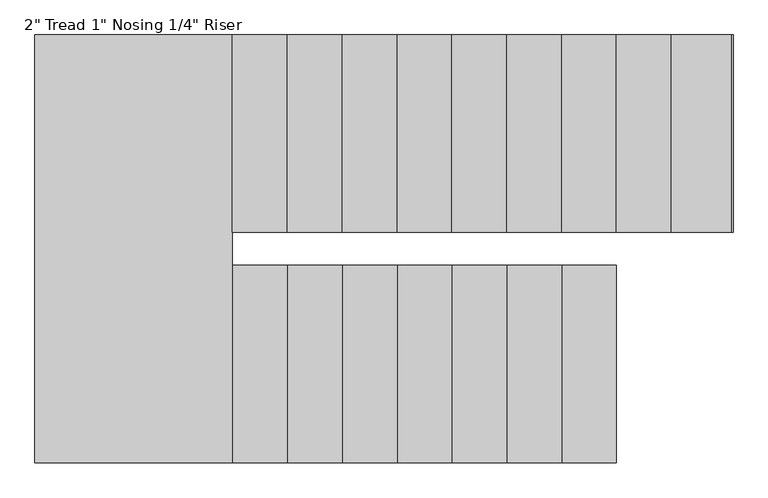
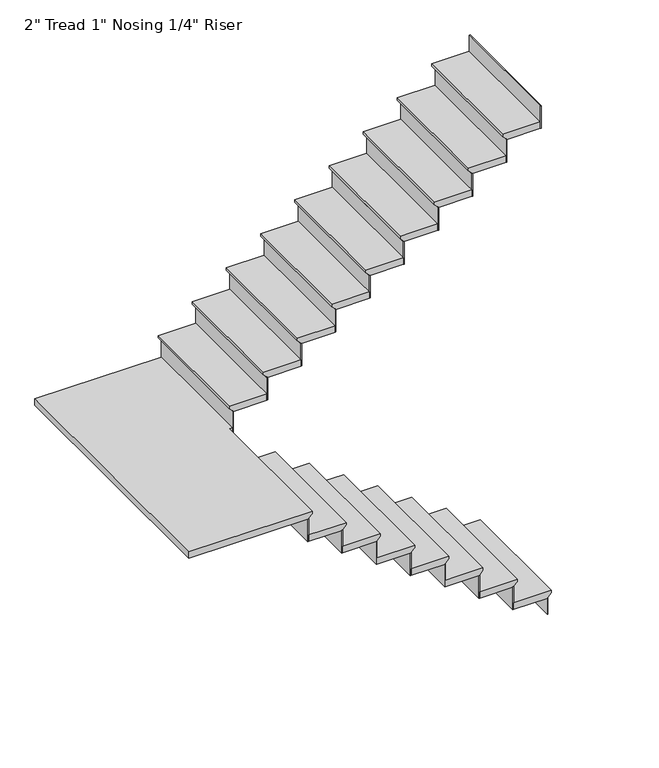
"""IFC4 building model written with IfcOpenShell, lengths in millimetres: stair flight geometry."""

from ifc_helpers import new_model, si_unit, origin, place, context, project, spatial, faceted_brep, source, transform, mapped, element, save


def stair_flight_30e1afdc(model_context):
    return source(origin(), model_context, "Body", "Brep", [
        faceted_brep([(-5739.8201068, -2431.6122986, 158.75), (-5739.8201068, -2431.6122986, 177.8), (-5739.8201068, -3346.0122986, 177.8), (-5739.8201068, -3346.0122986, 158.75), (-5765.2201068, -2431.6122986, 133.35), (-5765.2201068, -3346.0122986, 133.35), (-6019.2201068, -2431.6122986, 177.8), (-6019.2201068, -3346.0122986, 177.8), (-5765.2201068, -3346.0122986, 127.0), (-6019.2201068, -3346.0122986, 127.0), (-6019.2201068, -2431.6122986, 127.0), (-5765.2201068, -2431.6122986, 127.0)], [[[0, 1, 2, 3]], [[4, 0, 3, 5]], [[2, 1, 6, 7]], [[8, 9, 10, 11]], [[2, 7, 9, 8, 5, 3]], [[8, 11, 4, 5]], [[6, 1, 0, 4, 11, 10]], [[7, 6, 10, 9]]]),
        faceted_brep([(-5765.2201068, -2431.6122986, 127.0), (-5765.2201068, -2431.6122986, 0.0), (-5771.5701068, -2431.6122986, 0.0), (-5771.5701068, -2431.6122986, 127.0), (-5765.2201068, -3346.0122986, 127.0), (-5771.5701068, -3346.0122986, 127.0), (-5771.5701068, -3346.0122986, 0.0), (-5765.2201068, -3346.0122986, 0.0)], [[[0, 1, 2, 3]], [[4, 5, 6, 7]], [[1, 0, 4, 7]], [[2, 1, 7, 6]], [[3, 2, 6, 5]], [[0, 3, 5, 4]]]),
        faceted_brep([(-6019.2201068, -2431.6122986, 304.8), (-6019.2201068, -2431.6122986, 127.0), (-6025.5701068, -2431.6122986, 127.0), (-6025.5701068, -2431.6122986, 304.8), (-6019.2201068, -3346.0122986, 304.8), (-6025.5701068, -3346.0122986, 304.8), (-6025.5701068, -3346.0122986, 127.0), (-6019.2201068, -3346.0122986, 127.0)], [[[0, 1, 2, 3]], [[4, 5, 6, 7]], [[1, 0, 4, 7]], [[2, 1, 7, 6]], [[3, 2, 6, 5]], [[0, 3, 5, 4]]]),
        faceted_brep([(-5993.8201068, -3346.0122986, 355.6), (-5993.8201068, -2431.6122986, 355.6), (-6273.2201068, -2431.6122986, 355.6), (-6273.2201068, -3346.0122986, 355.6), (-6019.2201068, -3346.0122986, 304.8), (-6273.2201068, -3346.0122986, 304.8), (-6273.2201068, -2431.6122986, 304.8), (-6019.2201068, -2431.6122986, 304.8), (-6019.2201068, -3346.0122986, 311.15), (-5993.8201068, -3346.0122986, 336.55), (-6019.2201068, -2431.6122986, 311.15), (-5993.8201068, -2431.6122986, 336.55)], [[[0, 1, 2, 3]], [[4, 5, 6, 7]], [[0, 3, 5, 4, 8, 9]], [[4, 7, 10, 8]], [[2, 1, 11, 10, 7, 6]], [[3, 2, 6, 5]], [[11, 1, 0, 9]], [[10, 11, 9, 8]]]),
        faceted_brep([(-6273.2201068, -2431.6122986, 482.6), (-6273.2201068, -2431.6122986, 304.8), (-6279.5701068, -2431.6122986, 304.8), (-6279.5701068, -2431.6122986, 482.6), (-6273.2201068, -3346.0122986, 482.6), (-6279.5701068, -3346.0122986, 482.6), (-6279.5701068, -3346.0122986, 304.8), (-6273.2201068, -3346.0122986, 304.8)], [[[0, 1, 2, 3]], [[4, 5, 6, 7]], [[1, 0, 4, 7]], [[2, 1, 7, 6]], [[3, 2, 6, 5]], [[0, 3, 5, 4]]]),
        faceted_brep([(-6247.8201068, -3346.0122986, 533.4), (-6247.8201068, -2431.6122986, 533.4), (-6527.2201068, -2431.6122986, 533.4), (-6527.2201068, -3346.0122986, 533.4), (-6273.2201068, -3346.0122986, 482.6), (-6527.2201068, -3346.0122986, 482.6), (-6527.2201068, -2431.6122986, 482.6), (-6273.2201068, -2431.6122986, 482.6), (-6273.2201068, -3346.0122986, 488.95), (-6247.8201068, -3346.0122986, 514.35), (-6273.2201068, -2431.6122986, 488.95), (-6247.8201068, -2431.6122986, 514.35)], [[[0, 1, 2, 3]], [[4, 5, 6, 7]], [[0, 3, 5, 4, 8, 9]], [[4, 7, 10, 8]], [[2, 1, 11, 10, 7, 6]], [[3, 2, 6, 5]], [[11, 1, 0, 9]], [[10, 11, 9, 8]]]),
        faceted_brep([(-6527.2201068, -2431.6122986, 660.4), (-6527.2201068, -2431.6122986, 482.6), (-6533.5701068, -2431.6122986, 482.6), (-6533.5701068, -2431.6122986, 660.4), (-6527.2201068, -3346.0122986, 660.4), (-6533.5701068, -3346.0122986, 660.4), (-6533.5701068, -3346.0122986, 482.6), (-6527.2201068, -3346.0122986, 482.6)], [[[0, 1, 2, 3]], [[4, 5, 6, 7]], [[1, 0, 4, 7]], [[2, 1, 7, 6]], [[3, 2, 6, 5]], [[0, 3, 5, 4]]]),
        faceted_brep([(-6501.8201068, -3346.0122986, 711.2), (-6501.8201068, -2431.6122986, 711.2), (-6781.2201068, -2431.6122986, 711.2), (-6781.2201068, -3346.0122986, 711.2), (-6527.2201068, -3346.0122986, 660.4), (-6781.2201068, -3346.0122986, 660.4), (-6781.2201068, -2431.6122986, 660.4), (-6527.2201068, -2431.6122986, 660.4), (-6527.2201068, -3346.0122986, 666.75), (-6501.8201068, -3346.0122986, 692.15), (-6527.2201068, -2431.6122986, 666.75), (-6501.8201068, -2431.6122986, 692.15)], [[[0, 1, 2, 3]], [[4, 5, 6, 7]], [[0, 3, 5, 4, 8, 9]], [[4, 7, 10, 8]], [[2, 1, 11, 10, 7, 6]], [[3, 2, 6, 5]], [[11, 1, 0, 9]], [[10, 11, 9, 8]]]),
        faceted_brep([(-6781.2201068, -2431.6122986, 838.2), (-6781.2201068, -2431.6122986, 660.4), (-6787.5701068, -2431.6122986, 660.4), (-6787.5701068, -2431.6122986, 838.2), (-6781.2201068, -3346.0122986, 838.2), (-6787.5701068, -3346.0122986, 838.2), (-6787.5701068, -3346.0122986, 660.4), (-6781.2201068, -3346.0122986, 660.4)], [[[0, 1, 2, 3]], [[4, 5, 6, 7]], [[1, 0, 4, 7]], [[2, 1, 7, 6]], [[3, 2, 6, 5]], [[0, 3, 5, 4]]]),
        faceted_brep([(-6755.8201068, -3346.0122986, 889.0), (-6755.8201068, -2431.6122986, 889.0), (-7035.2201068, -2431.6122986, 889.0), (-7035.2201068, -3346.0122986, 889.0), (-6781.2201068, -3346.0122986, 838.2), (-7035.2201068, -3346.0122986, 838.2), (-7035.2201068, -2431.6122986, 838.2), (-6781.2201068, -2431.6122986, 838.2), (-6781.2201068, -3346.0122986, 844.55), (-6755.8201068, -3346.0122986, 869.95), (-6781.2201068, -2431.6122986, 844.55), (-6755.8201068, -2431.6122986, 869.95)], [[[0, 1, 2, 3]], [[4, 5, 6, 7]], [[0, 3, 5, 4, 8, 9]], [[4, 7, 10, 8]], [[2, 1, 11, 10, 7, 6]], [[3, 2, 6, 5]], [[11, 1, 0, 9]], [[10, 11, 9, 8]]]),
        faceted_brep([(-7035.2201068, -2431.6122986, 1016.0), (-7035.2201068, -2431.6122986, 838.2), (-7041.5701068, -2431.6122986, 838.2), (-7041.5701068, -2431.6122986, 1016.0), (-7035.2201068, -3346.0122986, 1016.0), (-7041.5701068, -3346.0122986, 1016.0), (-7041.5701068, -3346.0122986, 838.2), (-7035.2201068, -3346.0122986, 838.2)], [[[0, 1, 2, 3]], [[4, 5, 6, 7]], [[1, 0, 4, 7]], [[2, 1, 7, 6]], [[3, 2, 6, 5]], [[0, 3, 5, 4]]]),
        faceted_brep([(-7009.8201068, -3346.0122986, 1066.8), (-7009.8201068, -2431.6122986, 1066.8), (-7289.2201068, -2431.6122986, 1066.8), (-7289.2201068, -3346.0122986, 1066.8), (-7035.2201068, -3346.0122986, 1016.0), (-7289.2201068, -3346.0122986, 1016.0), (-7289.2201068, -2431.6122986, 1016.0), (-7035.2201068, -2431.6122986, 1016.0), (-7035.2201068, -3346.0122986, 1022.35), (-7009.8201068, -3346.0122986, 1047.75), (-7035.2201068, -2431.6122986, 1022.35), (-7009.8201068, -2431.6122986, 1047.75)], [[[0, 1, 2, 3]], [[4, 5, 6, 7]], [[0, 3, 5, 4, 8, 9]], [[4, 7, 10, 8]], [[2, 1, 11, 10, 7, 6]], [[3, 2, 6, 5]], [[11, 1, 0, 9]], [[10, 11, 9, 8]]]),
        faceted_brep([(-7543.2201068, -2431.6122986, 1371.6), (-7543.2201068, -2431.6122986, 1193.8), (-7549.5701068, -2431.6122986, 1193.8), (-7549.5701068, -2431.6122986, 1371.6), (-7543.2201068, -3346.0122986, 1371.6), (-7549.5701068, -3346.0122986, 1371.6), (-7549.5701068, -3346.0122986, 1193.8), (-7543.2201068, -3346.0122986, 1193.8)], [[[0, 1, 2, 3]], [[4, 5, 6, 7]], [[1, 0, 4, 7]], [[2, 1, 7, 6]], [[3, 2, 6, 5]], [[0, 3, 5, 4]]]),
        faceted_brep([(-7492.4201068, -1364.8122986, 1422.4), (-8432.2201068, -1364.8122986, 1422.4), (-8432.2201068, -3346.0122986, 1422.4), (-7517.8201068, -3346.0122986, 1422.4), (-7517.8201068, -2279.2122986, 1422.4), (-7492.4201068, -2279.2122986, 1422.4), (-8432.2201068, -1364.8122986, 1371.6), (-7492.4201068, -1364.8122986, 1371.6), (-7492.4201068, -2279.2122986, 1371.6), (-7517.8201068, -2279.2122986, 1371.6), (-7517.8201068, -2431.6122986, 1371.6), (-7543.2201068, -2431.6122986, 1371.6), (-7543.2201068, -3346.0122986, 1371.6), (-8432.2201068, -3346.0122986, 1371.6), (-7543.2201068, -2431.6122986, 1377.95), (-7543.2201068, -3346.0122986, 1377.95), (-7517.8201068, -3346.0122986, 1403.35), (-7517.8201068, -2431.6122986, 1403.35)], [[[0, 1, 2, 3, 4, 5]], [[6, 7, 8, 9, 10, 11, 12, 13]], [[1, 0, 7, 6]], [[12, 11, 14, 15]], [[4, 3, 16, 17, 10, 9]], [[0, 5, 8, 7]], [[16, 15, 14, 17]], [[2, 1, 6, 13]], [[3, 2, 13, 12, 15, 16]], [[11, 10, 17, 14]], [[5, 4, 9, 8]]]),
        faceted_brep([(-7289.2201068, -2431.6122986, 1193.8), (-7289.2201068, -2431.6122986, 1016.0), (-7295.5701068, -2431.6122986, 1016.0), (-7295.5701068, -2431.6122986, 1193.8), (-7289.2201068, -3346.0122986, 1193.8), (-7295.5701068, -3346.0122986, 1193.8), (-7295.5701068, -3346.0122986, 1016.0), (-7289.2201068, -3346.0122986, 1016.0)], [[[0, 1, 2, 3]], [[4, 5, 6, 7]], [[1, 0, 4, 7]], [[2, 1, 7, 6]], [[3, 2, 6, 5]], [[0, 3, 5, 4]]]),
        faceted_brep([(-7263.8201068, -3346.0122986, 1244.6), (-7263.8201068, -2431.6122986, 1244.6), (-7543.2201068, -2431.6122986, 1244.6), (-7543.2201068, -3346.0122986, 1244.6), (-7289.2201068, -3346.0122986, 1193.8), (-7543.2201068, -3346.0122986, 1193.8), (-7543.2201068, -2431.6122986, 1193.8), (-7289.2201068, -2431.6122986, 1193.8), (-7289.2201068, -3346.0122986, 1200.15), (-7263.8201068, -3346.0122986, 1225.55), (-7289.2201068, -2431.6122986, 1200.15), (-7263.8201068, -2431.6122986, 1225.55)], [[[0, 1, 2, 3]], [[4, 5, 6, 7]], [[0, 3, 5, 4, 8, 9]], [[4, 7, 10, 8]], [[2, 1, 11, 10, 7, 6]], [[3, 2, 6, 5]], [[11, 1, 0, 9]], [[10, 11, 9, 8]]]),
        faceted_brep([(-7492.4201068, -2279.2122986, 1549.4), (-7492.4201068, -2279.2122986, 1371.6), (-7486.0701068, -2279.2122986, 1371.6), (-7486.0701068, -2279.2122986, 1549.4), (-7492.4201068, -1364.8122986, 1549.4), (-7486.0701068, -1364.8122986, 1549.4), (-7486.0701068, -1364.8122986, 1371.6), (-7492.4201068, -1364.8122986, 1371.6)], [[[0, 1, 2, 3]], [[4, 5, 6, 7]], [[1, 0, 4, 7]], [[2, 1, 7, 6]], [[3, 2, 6, 5]], [[0, 3, 5, 4]]]),
        faceted_brep([(-7517.8201068, -1364.8122986, 1600.2), (-7517.8201068, -2279.2122986, 1600.2), (-7238.4201068, -2279.2122986, 1600.2), (-7238.4201068, -1364.8122986, 1600.2), (-7492.4201068, -1364.8122986, 1549.4), (-7238.4201068, -1364.8122986, 1549.4), (-7238.4201068, -2279.2122986, 1549.4), (-7492.4201068, -2279.2122986, 1549.4), (-7492.4201068, -1364.8122986, 1555.75), (-7517.8201068, -1364.8122986, 1581.15), (-7492.4201068, -2279.2122986, 1555.75), (-7517.8201068, -2279.2122986, 1581.15)], [[[0, 1, 2, 3]], [[4, 5, 6, 7]], [[0, 3, 5, 4, 8, 9]], [[4, 7, 10, 8]], [[2, 1, 11, 10, 7, 6]], [[3, 2, 6, 5]], [[11, 1, 0, 9]], [[10, 11, 9, 8]]]),
        faceted_brep([(-7238.4201068, -2279.2122986, 1727.2), (-7238.4201068, -2279.2122986, 1549.4), (-7232.0701068, -2279.2122986, 1549.4), (-7232.0701068, -2279.2122986, 1727.2), (-7238.4201068, -1364.8122986, 1727.2), (-7232.0701068, -1364.8122986, 1727.2), (-7232.0701068, -1364.8122986, 1549.4), (-7238.4201068, -1364.8122986, 1549.4)], [[[0, 1, 2, 3]], [[4, 5, 6, 7]], [[1, 0, 4, 7]], [[2, 1, 7, 6]], [[3, 2, 6, 5]], [[0, 3, 5, 4]]]),
        faceted_brep([(-7263.8201068, -1364.8122986, 1778.0), (-7263.8201068, -2279.2122986, 1778.0), (-6984.4201068, -2279.2122986, 1778.0), (-6984.4201068, -1364.8122986, 1778.0), (-7238.4201068, -1364.8122986, 1727.2), (-6984.4201068, -1364.8122986, 1727.2), (-6984.4201068, -2279.2122986, 1727.2), (-7238.4201068, -2279.2122986, 1727.2), (-7238.4201068, -1364.8122986, 1733.55), (-7263.8201068, -1364.8122986, 1758.95), (-7238.4201068, -2279.2122986, 1733.55), (-7263.8201068, -2279.2122986, 1758.95)], [[[0, 1, 2, 3]], [[4, 5, 6, 7]], [[0, 3, 5, 4, 8, 9]], [[4, 7, 10, 8]], [[2, 1, 11, 10, 7, 6]], [[3, 2, 6, 5]], [[11, 1, 0, 9]], [[10, 11, 9, 8]]]),
        faceted_brep([(-6984.4201068, -2279.2122986, 1905.0), (-6984.4201068, -2279.2122986, 1727.2), (-6978.0701068, -2279.2122986, 1727.2), (-6978.0701068, -2279.2122986, 1905.0), (-6984.4201068, -1364.8122986, 1905.0), (-6978.0701068, -1364.8122986, 1905.0), (-6978.0701068, -1364.8122986, 1727.2), (-6984.4201068, -1364.8122986, 1727.2)], [[[0, 1, 2, 3]], [[4, 5, 6, 7]], [[1, 0, 4, 7]], [[2, 1, 7, 6]], [[3, 2, 6, 5]], [[0, 3, 5, 4]]]),
        faceted_brep([(-7009.8201068, -1364.8122986, 1955.8), (-7009.8201068, -2279.2122986, 1955.8), (-6730.4201068, -2279.2122986, 1955.8), (-6730.4201068, -1364.8122986, 1955.8), (-6984.4201068, -1364.8122986, 1905.0), (-6730.4201068, -1364.8122986, 1905.0), (-6730.4201068, -2279.2122986, 1905.0), (-6984.4201068, -2279.2122986, 1905.0), (-6984.4201068, -1364.8122986, 1911.35), (-7009.8201068, -1364.8122986, 1936.75), (-6984.4201068, -2279.2122986, 1911.35), (-7009.8201068, -2279.2122986, 1936.75)], [[[0, 1, 2, 3]], [[4, 5, 6, 7]], [[0, 3, 5, 4, 8, 9]], [[4, 7, 10, 8]], [[2, 1, 11, 10, 7, 6]], [[3, 2, 6, 5]], [[11, 1, 0, 9]], [[10, 11, 9, 8]]]),
        faceted_brep([(-6730.4201068, -2279.2122986, 2082.8), (-6730.4201068, -2279.2122986, 1905.0), (-6724.0701068, -2279.2122986, 1905.0), (-6724.0701068, -2279.2122986, 2082.8), (-6730.4201068, -1364.8122986, 2082.8), (-6724.0701068, -1364.8122986, 2082.8), (-6724.0701068, -1364.8122986, 1905.0), (-6730.4201068, -1364.8122986, 1905.0)], [[[0, 1, 2, 3]], [[4, 5, 6, 7]], [[1, 0, 4, 7]], [[2, 1, 7, 6]], [[3, 2, 6, 5]], [[0, 3, 5, 4]]]),
        faceted_brep([(-6755.8201068, -1364.8122986, 2133.6), (-6755.8201068, -2279.2122986, 2133.6), (-6476.4201068, -2279.2122986, 2133.6), (-6476.4201068, -1364.8122986, 2133.6), (-6730.4201068, -1364.8122986, 2082.8), (-6476.4201068, -1364.8122986, 2082.8), (-6476.4201068, -2279.2122986, 2082.8), (-6730.4201068, -2279.2122986, 2082.8), (-6730.4201068, -1364.8122986, 2089.15), (-6755.8201068, -1364.8122986, 2114.55), (-6730.4201068, -2279.2122986, 2089.15), (-6755.8201068, -2279.2122986, 2114.55)], [[[0, 1, 2, 3]], [[4, 5, 6, 7]], [[0, 3, 5, 4, 8, 9]], [[4, 7, 10, 8]], [[2, 1, 11, 10, 7, 6]], [[3, 2, 6, 5]], [[11, 1, 0, 9]], [[10, 11, 9, 8]]]),
        faceted_brep([(-6476.4201068, -2279.2122986, 2260.6), (-6476.4201068, -2279.2122986, 2082.8), (-6470.0701068, -2279.2122986, 2082.8), (-6470.0701068, -2279.2122986, 2260.6), (-6476.4201068, -1364.8122986, 2260.6), (-6470.0701068, -1364.8122986, 2260.6), (-6470.0701068, -1364.8122986, 2082.8), (-6476.4201068, -1364.8122986, 2082.8)], [[[0, 1, 2, 3]], [[4, 5, 6, 7]], [[1, 0, 4, 7]], [[2, 1, 7, 6]], [[3, 2, 6, 5]], [[0, 3, 5, 4]]]),
        faceted_brep([(-6501.8201068, -1364.8122986, 2311.4), (-6501.8201068, -2279.2122986, 2311.4), (-6222.4201068, -2279.2122986, 2311.4), (-6222.4201068, -1364.8122986, 2311.4), (-6476.4201068, -1364.8122986, 2260.6), (-6222.4201068, -1364.8122986, 2260.6), (-6222.4201068, -2279.2122986, 2260.6), (-6476.4201068, -2279.2122986, 2260.6), (-6476.4201068, -1364.8122986, 2266.95), (-6501.8201068, -1364.8122986, 2292.35), (-6476.4201068, -2279.2122986, 2266.95), (-6501.8201068, -2279.2122986, 2292.35)], [[[0, 1, 2, 3]], [[4, 5, 6, 7]], [[0, 3, 5, 4, 8, 9]], [[4, 7, 10, 8]], [[2, 1, 11, 10, 7, 6]], [[3, 2, 6, 5]], [[11, 1, 0, 9]], [[10, 11, 9, 8]]]),
        faceted_brep([(-6222.4201068, -2279.2122986, 2438.4), (-6222.4201068, -2279.2122986, 2260.6), (-6216.0701068, -2279.2122986, 2260.6), (-6216.0701068, -2279.2122986, 2438.4), (-6222.4201068, -1364.8122986, 2438.4), (-6216.0701068, -1364.8122986, 2438.4), (-6216.0701068, -1364.8122986, 2260.6), (-6222.4201068, -1364.8122986, 2260.6)], [[[0, 1, 2, 3]], [[4, 5, 6, 7]], [[1, 0, 4, 7]], [[2, 1, 7, 6]], [[3, 2, 6, 5]], [[0, 3, 5, 4]]]),
        faceted_brep([(-6247.8201068, -1364.8122986, 2489.2), (-6247.8201068, -2279.2122986, 2489.2), (-5968.4201068, -2279.2122986, 2489.2), (-5968.4201068, -1364.8122986, 2489.2), (-6222.4201068, -1364.8122986, 2438.4), (-5968.4201068, -1364.8122986, 2438.4), (-5968.4201068, -2279.2122986, 2438.4), (-6222.4201068, -2279.2122986, 2438.4), (-6222.4201068, -1364.8122986, 2444.75), (-6247.8201068, -1364.8122986, 2470.15), (-6222.4201068, -2279.2122986, 2444.75), (-6247.8201068, -2279.2122986, 2470.15)], [[[0, 1, 2, 3]], [[4, 5, 6, 7]], [[0, 3, 5, 4, 8, 9]], [[4, 7, 10, 8]], [[2, 1, 11, 10, 7, 6]], [[3, 2, 6, 5]], [[11, 1, 0, 9]], [[10, 11, 9, 8]]]),
        faceted_brep([(-5968.4201068, -2279.2122986, 2616.2), (-5968.4201068, -2279.2122986, 2438.4), (-5962.0701068, -2279.2122986, 2438.4), (-5962.0701068, -2279.2122986, 2616.2), (-5968.4201068, -1364.8122986, 2616.2), (-5962.0701068, -1364.8122986, 2616.2), (-5962.0701068, -1364.8122986, 2438.4), (-5968.4201068, -1364.8122986, 2438.4)], [[[0, 1, 2, 3]], [[4, 5, 6, 7]], [[1, 0, 4, 7]], [[2, 1, 7, 6]], [[3, 2, 6, 5]], [[0, 3, 5, 4]]]),
        faceted_brep([(-5993.8201068, -1364.8122986, 2667.0), (-5993.8201068, -2279.2122986, 2667.0), (-5714.4201068, -2279.2122986, 2667.0), (-5714.4201068, -1364.8122986, 2667.0), (-5968.4201068, -1364.8122986, 2616.2), (-5714.4201068, -1364.8122986, 2616.2), (-5714.4201068, -2279.2122986, 2616.2), (-5968.4201068, -2279.2122986, 2616.2), (-5968.4201068, -1364.8122986, 2622.55), (-5993.8201068, -1364.8122986, 2647.95), (-5968.4201068, -2279.2122986, 2622.55), (-5993.8201068, -2279.2122986, 2647.95)], [[[0, 1, 2, 3]], [[4, 5, 6, 7]], [[0, 3, 5, 4, 8, 9]], [[4, 7, 10, 8]], [[2, 1, 11, 10, 7, 6]], [[3, 2, 6, 5]], [[11, 1, 0, 9]], [[10, 11, 9, 8]]]),
        faceted_brep([(-5714.4201068, -2279.2122986, 2794.0), (-5714.4201068, -2279.2122986, 2616.2), (-5708.0701068, -2279.2122986, 2616.2), (-5708.0701068, -2279.2122986, 2794.0), (-5714.4201068, -1364.8122986, 2794.0), (-5708.0701068, -1364.8122986, 2794.0), (-5708.0701068, -1364.8122986, 2616.2), (-5714.4201068, -1364.8122986, 2616.2)], [[[0, 1, 2, 3]], [[4, 5, 6, 7]], [[1, 0, 4, 7]], [[2, 1, 7, 6]], [[3, 2, 6, 5]], [[0, 3, 5, 4]]]),
        faceted_brep([(-5739.8201068, -1364.8122986, 2844.8), (-5739.8201068, -2279.2122986, 2844.8), (-5460.4201068, -2279.2122986, 2844.8), (-5460.4201068, -1364.8122986, 2844.8), (-5714.4201068, -1364.8122986, 2794.0), (-5460.4201068, -1364.8122986, 2794.0), (-5460.4201068, -2279.2122986, 2794.0), (-5714.4201068, -2279.2122986, 2794.0), (-5714.4201068, -1364.8122986, 2800.35), (-5739.8201068, -1364.8122986, 2825.75), (-5714.4201068, -2279.2122986, 2800.35), (-5739.8201068, -2279.2122986, 2825.75)], [[[0, 1, 2, 3]], [[4, 5, 6, 7]], [[0, 3, 5, 4, 8, 9]], [[4, 7, 10, 8]], [[2, 1, 11, 10, 7, 6]], [[3, 2, 6, 5]], [[11, 1, 0, 9]], [[10, 11, 9, 8]]]),
        faceted_brep([(-5460.4201068, -2279.2122986, 2971.8), (-5460.4201068, -2279.2122986, 2794.0), (-5454.0701068, -2279.2122986, 2794.0), (-5454.0701068, -2279.2122986, 2971.8), (-5460.4201068, -1364.8122986, 2971.8), (-5454.0701068, -1364.8122986, 2971.8), (-5454.0701068, -1364.8122986, 2794.0), (-5460.4201068, -1364.8122986, 2794.0)], [[[0, 1, 2, 3]], [[4, 5, 6, 7]], [[1, 0, 4, 7]], [[2, 1, 7, 6]], [[3, 2, 6, 5]], [[0, 3, 5, 4]]]),
        faceted_brep([(-5206.4201068, -2279.2122986, 3149.6), (-5206.4201068, -2279.2122986, 2971.8), (-5200.0701068, -2279.2122986, 2971.8), (-5200.0701068, -2279.2122986, 3149.6), (-5206.4201068, -1364.8122986, 3149.6), (-5200.0701068, -1364.8122986, 3149.6), (-5200.0701068, -1364.8122986, 2971.8), (-5206.4201068, -1364.8122986, 2971.8)], [[[0, 1, 2, 3]], [[4, 5, 6, 7]], [[1, 0, 4, 7]], [[2, 1, 7, 6]], [[3, 2, 6, 5]], [[0, 3, 5, 4]]]),
        faceted_brep([(-5485.8201068, -1364.8122986, 3022.6), (-5485.8201068, -2279.2122986, 3022.6), (-5206.4201068, -2279.2122986, 3022.6), (-5206.4201068, -1364.8122986, 3022.6), (-5460.4201068, -1364.8122986, 2971.8), (-5206.4201068, -1364.8122986, 2971.8), (-5206.4201068, -2279.2122986, 2971.8), (-5460.4201068, -2279.2122986, 2971.8), (-5460.4201068, -1364.8122986, 2978.15), (-5485.8201068, -1364.8122986, 3003.55), (-5460.4201068, -2279.2122986, 2978.15), (-5485.8201068, -2279.2122986, 3003.55)], [[[0, 1, 2, 3]], [[4, 5, 6, 7]], [[0, 3, 5, 4, 8, 9]], [[4, 7, 10, 8]], [[2, 1, 11, 10, 7, 6]], [[3, 2, 6, 5]], [[11, 1, 0, 9]], [[10, 11, 9, 8]]]),
    ])


if __name__ == "__main__":
    model = new_model("IFC4")
    model_context = context("Model", 3, world=origin())
    ifc_project = project(units=[si_unit("LENGTHUNIT", "METRE", prefix="MILLI")], contexts=[model_context])
    site = spatial("IfcSite", under=ifc_project)
    building = spatial("IfcBuilding", under=site)
    placement = place(None, origin())
    stair_flight_shape = stair_flight_30e1afdc(model_context)
    element("IfcStairFlight", 1, ObjectType="2\" Tread 1\" Nosing 1/4\" Riser", at=placement, inside=building, context=model_context, shape_type="MappedRepresentation", body=[
        mapped(stair_flight_shape, transform((0.0, 0.0, 0.0), x_axis=(1.0, 0.0, 0.0), y_axis=(0.0, 1.0, 0.0), z_axis=(0.0, 0.0, 1.0))),
    ])
    save(model, "model.ifc")

# Revit data of these elements
# Element 1 (IfcStairFlight, "2\" Tread 1\" Nosing 1/4\" Riser")
#   Materials on its faces: "0 olive green"
# Materials
#   "0 olive green": class "Generic", colour RGB 120 120 120, transparency 0, Cost = 0
